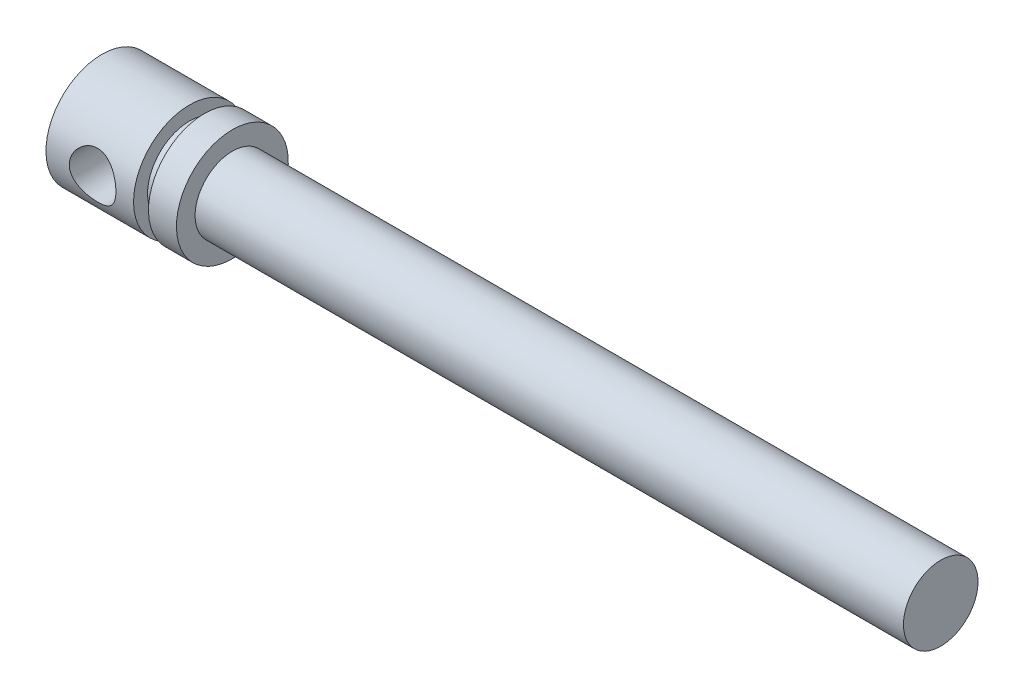
ISO-10303-21;
HEADER;
FILE_DESCRIPTION(('STEP AP214'),'2;1');
FILE_NAME('part.step','',(''),(''),'','','');
FILE_SCHEMA(('AUTOMOTIVE_DESIGN { 1 0 10303 214 1 1 1 1 }'));
ENDSEC;
DATA;
#1=APPLICATION_CONTEXT('core data for automotive mechanical design processes');
#2=APPLICATION_PROTOCOL_DEFINITION('international standard','automotive_design',2000,#1);
#3=PRODUCT_CONTEXT('',#1,'mechanical');
#4=PRODUCT('Part','Part','',(#3));
#5=PRODUCT_RELATED_PRODUCT_CATEGORY('part','',(#4));
#6=PRODUCT_DEFINITION_FORMATION('','',#4);
#7=PRODUCT_DEFINITION_CONTEXT('part definition',#1,'design');
#8=PRODUCT_DEFINITION('design','',#6,#7);
#9=PRODUCT_DEFINITION_SHAPE('','',#8);
#10=(LENGTH_UNIT() NAMED_UNIT(*) SI_UNIT(.MILLI.,.METRE.));
#11=(NAMED_UNIT(*) PLANE_ANGLE_UNIT() SI_UNIT($,.RADIAN.));
#12=(NAMED_UNIT(*) SI_UNIT($,.STERADIAN.) SOLID_ANGLE_UNIT());
#13=UNCERTAINTY_MEASURE_WITH_UNIT(LENGTH_MEASURE(1.E-05),#10,'distance_accuracy_value','');
#14=(GEOMETRIC_REPRESENTATION_CONTEXT(3) GLOBAL_UNCERTAINTY_ASSIGNED_CONTEXT((#13)) GLOBAL_UNIT_ASSIGNED_CONTEXT((#10,
#11,#12)) REPRESENTATION_CONTEXT('',''));
#15=CARTESIAN_POINT('',(0.,0.,0.));
#16=DIRECTION('',(0.,0.,1.));
#17=DIRECTION('',(1.,0.,0.));
#18=AXIS2_PLACEMENT_3D('',#15,#16,#17);
#19=CARTESIAN_POINT('',(0.,0.,0.));
#20=DIRECTION('',(-1.,0.,0.));
#21=DIRECTION('',(0.,-1.,0.));
#22=AXIS2_PLACEMENT_3D('',#19,#20,#21);
#23=PLANE('',#22);
#24=CARTESIAN_POINT('',(0.,0.,0.));
#25=DIRECTION('',(1.,0.,0.));
#26=DIRECTION('',(0.,1.,0.));
#27=AXIS2_PLACEMENT_3D('',#24,#25,#26);
#28=CIRCLE('',#27,6.);
#29=CARTESIAN_POINT('',(0.,6.,0.));
#30=VERTEX_POINT('',#29);
#31=EDGE_CURVE('E51',#30,#30,#28,.T.);
#32=ORIENTED_EDGE('',*,*,#31,.F.);
#33=EDGE_LOOP('',(#32));
#34=FACE_BOUND('',#33,.T.);
#35=ADVANCED_FACE('F40',(#34),#23,.T.);
#36=CARTESIAN_POINT('',(90.,0.,0.));
#37=DIRECTION('',(1.,0.,0.));
#38=DIRECTION('',(0.,1.,0.));
#39=AXIS2_PLACEMENT_3D('',#36,#37,#38);
#40=CYLINDRICAL_SURFACE('',#39,5.99999999999999);
#41=CARTESIAN_POINT('',(7.5,0.,-5.99999999999999));
#42=CARTESIAN_POINT('',(7.4999952878604,-0.133903918163791,-5.99999628290906));
#43=CARTESIAN_POINT('',(7.48917868439947,-0.268039524991424,-5.99546656821163));
#44=CARTESIAN_POINT('',(7.44631926190637,-0.532498019991114,-5.97780115788616));
#45=CARTESIAN_POINT('',(7.41422105321848,-0.66281002980867,-5.9646430059979));
#46=CARTESIAN_POINT('',(7.3301785119407,-0.915376593299225,-5.93112629106011));
#47=CARTESIAN_POINT('',(7.27830140767691,-1.03765681434384,-5.91079213642028));
#48=CARTESIAN_POINT('',(7.15645416697814,-1.27165974779733,-5.86490559253449));
#49=CARTESIAN_POINT('',(7.08648951102523,-1.38338564416287,-5.83935478441346));
#50=CARTESIAN_POINT('',(6.92674208819245,-1.59889674004597,-5.78415660619863));
#51=CARTESIAN_POINT('',(6.83619739674829,-1.70208251703042,-5.75437507703431));
#52=CARTESIAN_POINT('',(6.63947131609954,-1.8923196601971,-5.69465427085227));
#53=CARTESIAN_POINT('',(6.53328174628491,-1.9793625312399,-5.66471491925557));
#54=CARTESIAN_POINT('',(6.30194644898946,-2.13907474876483,-5.60642043928223));
#55=CARTESIAN_POINT('',(6.17612510424857,-2.2108261616941,-5.57821573827598));
#56=CARTESIAN_POINT('',(5.91285348305705,-2.331878813161,-5.52871144633221));
#57=CARTESIAN_POINT('',(5.77540924074289,-2.38119161708799,-5.507408299805));
#58=CARTESIAN_POINT('',(5.49969261673848,-2.45349196589845,-5.47557110795536));
#59=CARTESIAN_POINT('',(5.36177903328898,-2.47763315746001,-5.4645677530895));
#60=CARTESIAN_POINT('',(5.08345341455361,-2.50250419944798,-5.45322652433632));
#61=CARTESIAN_POINT('',(4.94304279992962,-2.5032469611117,-5.45288276849132));
#62=CARTESIAN_POINT('',(4.67519987914757,-2.48216900725155,-5.46250239122984));
#63=CARTESIAN_POINT('',(4.54759780687576,-2.46207362224014,-5.47167765447588));
#64=CARTESIAN_POINT('',(4.29777581799454,-2.40278382032141,-5.49796965547248));
#65=CARTESIAN_POINT('',(4.17555693701519,-2.36358574574513,-5.51508791407033));
#66=CARTESIAN_POINT('',(3.93688459401841,-2.26643917454979,-5.55572369545607));
#67=CARTESIAN_POINT('',(3.82060915817359,-2.20810943078428,-5.57936963898297));
#68=CARTESIAN_POINT('',(3.59904453223936,-2.07462485161169,-5.63036662282145));
#69=CARTESIAN_POINT('',(3.49375969877287,-1.99946338103921,-5.65771912259551));
#70=CARTESIAN_POINT('',(3.28780008253443,-1.82699193108754,-5.71585953755965));
#71=CARTESIAN_POINT('',(3.18826686522916,-1.72834696641502,-5.74674242808946));
#72=CARTESIAN_POINT('',(3.00677299408161,-1.51545918210306,-5.80651346225055));
#73=CARTESIAN_POINT('',(2.92481645661564,-1.40121271889692,-5.83540113754018));
#74=CARTESIAN_POINT('',(2.77912835276747,-1.15689589738674,-5.88876567112945));
#75=CARTESIAN_POINT('',(2.71586110969864,-1.02652116489536,-5.91312533086666));
#76=CARTESIAN_POINT('',(2.61255772079348,-0.755704805053667,-5.95378962829605));
#77=CARTESIAN_POINT('',(2.57250873611237,-0.615268789590071,-5.97009871691599));
#78=CARTESIAN_POINT('',(2.51916801574673,-0.337856226692456,-5.99199282372769));
#79=CARTESIAN_POINT('',(2.5043442851125,-0.201222570557278,-5.99819082094249));
#80=CARTESIAN_POINT('',(2.49730755277181,0.0727093109921778,-6.00112100737489));
#81=CARTESIAN_POINT('',(2.505088059496,0.21000733430527,-5.99785591423877));
#82=CARTESIAN_POINT('',(2.54194216961213,0.474196484682871,-5.98262435313879));
#83=CARTESIAN_POINT('',(2.56993990819439,0.601265933278776,-5.97109774567978));
#84=CARTESIAN_POINT('',(2.64493638908157,0.848765497942179,-5.94097213544828));
#85=CARTESIAN_POINT('',(2.69193753190061,0.969194773036713,-5.92237223919407));
#86=CARTESIAN_POINT('',(2.80514195142423,1.20421799973828,-5.8791654129033));
#87=CARTESIAN_POINT('',(2.87189636629204,1.31851447371068,-5.8543898293856));
#88=CARTESIAN_POINT('',(3.02210675558342,1.53469243246282,-5.80147609158182));
#89=CARTESIAN_POINT('',(3.10556970305865,1.63656870520375,-5.77333653537472));
#90=CARTESIAN_POINT('',(3.29380646654471,1.83266686054867,-5.71424175790866));
#91=CARTESIAN_POINT('',(3.39967700597211,1.92582139596023,-5.68322903182027));
#92=CARTESIAN_POINT('',(3.6260425518712,2.09333969221046,-5.62368673536039));
#93=CARTESIAN_POINT('',(3.74654087034502,2.16769918571027,-5.59515772986986));
#94=CARTESIAN_POINT('',(4.00122835060358,2.2963192041761,-5.54362772487863));
#95=CARTESIAN_POINT('',(4.13558807102375,2.35027836475451,-5.52071125109801));
#96=CARTESIAN_POINT('',(4.41274118762612,2.43434827902353,-5.48416711318334));
#97=CARTESIAN_POINT('',(4.55552752498876,2.46447869724417,-5.47053179113072));
#98=CARTESIAN_POINT('',(4.83363739837805,2.49808160700532,-5.45526329073079));
#99=CARTESIAN_POINT('',(4.96868932451195,2.50342760836084,-5.45278701929113));
#100=CARTESIAN_POINT('',(5.23768572235548,2.49231151038,-5.45787706027258));
#101=CARTESIAN_POINT('',(5.3716303609001,2.47585275892879,-5.46544183100006));
#102=CARTESIAN_POINT('',(5.62818549467776,2.42316809595844,-5.48899102586043));
#103=CARTESIAN_POINT('',(5.75103334597753,2.38789807270203,-5.50456709625452));
#104=CARTESIAN_POINT('',(5.98909604366397,2.29952656276963,-5.54206362465903));
#105=CARTESIAN_POINT('',(6.10430873433601,2.24642006560089,-5.56398586515028));
#106=CARTESIAN_POINT('',(6.33139178814705,2.1202057237392,-5.61333908853253));
#107=CARTESIAN_POINT('',(6.44264464594781,2.04608723750136,-5.64102204404078));
#108=CARTESIAN_POINT('',(6.65172029311513,1.88136812596239,-5.69807379131313));
#109=CARTESIAN_POINT('',(6.74953840503241,1.79076178563715,-5.72744316520043));
#110=CARTESIAN_POINT('',(6.93629730561753,1.58780416898838,-5.78712781593092));
#111=CARTESIAN_POINT('',(7.0240726428278,1.47434977868814,-5.81735619175009));
#112=CARTESIAN_POINT('',(7.17939913004211,1.23319985958043,-5.87320303099821));
#113=CARTESIAN_POINT('',(7.24694106399683,1.1054978774169,-5.89881939160171));
#114=CARTESIAN_POINT('',(7.3584188704516,0.841465213422193,-5.94218308378895));
#115=CARTESIAN_POINT('',(7.40272649429008,0.705312056415867,-5.96005349044658));
#116=CARTESIAN_POINT('',(7.46741568752959,0.426816782070268,-5.98642234975889));
#117=CARTESIAN_POINT('',(7.48787216820581,0.284495506121989,-5.99495014042421));
#118=CARTESIAN_POINT('',(7.49732384178621,0.118052512349437,-5.99888566614291));
#119=CARTESIAN_POINT('',(7.49832660250302,0.0944569348794029,-5.99930292614997));
#120=CARTESIAN_POINT('',(7.49966509825678,0.0472433090693365,-5.99986042138655));
#121=CARTESIAN_POINT('',(7.50000083138364,0.0236252606651506,-6.00000065582279));
#122=CARTESIAN_POINT('',(7.5,0.,-5.99999999999999));
#123=B_SPLINE_CURVE_WITH_KNOTS('',3,(#41,#42,#43,#44,#45,#46,#47,#48,#49,#50,#51,#52,#53,#54,
#55,#56,#57,#58,#59,#60,#61,#62,#63,#64,#65,#66,#67,#68,#69,#70,#71,#72,#73,#74,#75,#76,#77,#78,
#79,#80,#81,#82,#83,#84,#85,#86,#87,#88,#89,#90,#91,#92,#93,#94,#95,#96,#97,#98,#99,#100,#101,
#102,#103,#104,#105,#106,#107,#108,#109,#110,#111,#112,#113,#114,#115,#116,#117,#118,#119,#120,
#121,#122),.UNSPECIFIED.,.T.,.F.,(4,2,2,2,2,2,2,2,2,2,2,2,2,2,2,2,2,2,2,2,2,2,2,2,2,2,2,2,2,2,2,
2,2,2,2,2,2,2,2,2,4),(0.,0.401613837767878,0.804277081257394,1.2055837038126,1.60676887370595,
2.02635872577614,2.44616876262931,2.88663449078251,3.32687293461176,3.74590546275115,
4.16470676498092,4.55140314405113,4.93817359454425,5.33317426117429,5.72833091434413,
6.15688282255793,6.58553498629176,7.02408110121627,7.46238448436594,7.87296886786502,
8.28343534986344,8.67353179471443,9.0636775320357,9.46594270544322,9.86837610938992,
10.2995697605859,10.7308612248068,11.1682957671905,11.6053689414916,12.0087975511929,
12.4121642259507,12.7967529992953,13.1814498990123,13.5892778679488,13.9972474685189,
14.4349307000978,14.8728129885717,15.3034571163877,15.7327450093864,15.8036033125922,
15.8744618187069),.UNSPECIFIED.);
#124=CARTESIAN_POINT('',(7.5,0.,-5.99999999999999));
#125=VERTEX_POINT('',#124);
#126=EDGE_CURVE('E10',#125,#125,#123,.T.);
#127=ORIENTED_EDGE('',*,*,#126,.F.);
#128=EDGE_LOOP('',(#127));
#129=FACE_BOUND('',#128,.T.);
#130=CARTESIAN_POINT('',(7.5,0.,6.));
#131=CARTESIAN_POINT('',(7.4999952878604,0.133903918163793,5.99999628290908));
#132=CARTESIAN_POINT('',(7.48917868439947,0.268039524991427,5.99546656821164));
#133=CARTESIAN_POINT('',(7.44631926190637,0.532498019991115,5.97780115788615));
#134=CARTESIAN_POINT('',(7.41422105321848,0.662810029808672,5.9646430059979));
#135=CARTESIAN_POINT('',(7.3301785119407,0.915376593299227,5.93112629106011));
#136=CARTESIAN_POINT('',(7.27830140767691,1.03765681434384,5.91079213642028));
#137=CARTESIAN_POINT('',(7.15645416697814,1.27165974779733,5.86490559253449));
#138=CARTESIAN_POINT('',(7.08648951102523,1.38338564416287,5.83935478441346));
#139=CARTESIAN_POINT('',(6.92674208819245,1.59889674004597,5.78415660619863));
#140=CARTESIAN_POINT('',(6.83619739674829,1.70208251703042,5.75437507703432));
#141=CARTESIAN_POINT('',(6.63947131609954,1.8923196601971,5.69465427085227));
#142=CARTESIAN_POINT('',(6.53328174628491,1.9793625312399,5.66471491925557));
#143=CARTESIAN_POINT('',(6.30194644898946,2.13907474876483,5.60642043928223));
#144=CARTESIAN_POINT('',(6.17612510424856,2.2108261616941,5.57821573827598));
#145=CARTESIAN_POINT('',(5.91285348305705,2.331878813161,5.52871144633221));
#146=CARTESIAN_POINT('',(5.77540924074289,2.38119161708799,5.507408299805));
#147=CARTESIAN_POINT('',(5.49969261673848,2.45349196589845,5.47557110795536));
#148=CARTESIAN_POINT('',(5.36177903328898,2.47763315746001,5.46456775308951));
#149=CARTESIAN_POINT('',(5.08345341455361,2.50250419944798,5.45322652433632));
#150=CARTESIAN_POINT('',(4.94304279992962,2.5032469611117,5.45288276849132));
#151=CARTESIAN_POINT('',(4.67519987914757,2.48216900725155,5.46250239122984));
#152=CARTESIAN_POINT('',(4.54759780687576,2.46207362224014,5.47167765447588));
#153=CARTESIAN_POINT('',(4.29777581799454,2.40278382032141,5.49796965547248));
#154=CARTESIAN_POINT('',(4.17555693701519,2.36358574574513,5.51508791407033));
#155=CARTESIAN_POINT('',(3.93688459401841,2.26643917454979,5.55572369545607));
#156=CARTESIAN_POINT('',(3.82060915817359,2.20810943078428,5.57936963898297));
#157=CARTESIAN_POINT('',(3.59904453223936,2.07462485161168,5.63036662282145));
#158=CARTESIAN_POINT('',(3.49375969877287,1.99946338103921,5.65771912259551));
#159=CARTESIAN_POINT('',(3.28780008253443,1.82699193108754,5.71585953755965));
#160=CARTESIAN_POINT('',(3.18826686522915,1.72834696641502,5.74674242808946));
#161=CARTESIAN_POINT('',(3.00677299408161,1.51545918210306,5.80651346225055));
#162=CARTESIAN_POINT('',(2.92481645661564,1.40121271889692,5.83540113754018));
#163=CARTESIAN_POINT('',(2.77912835276747,1.15689589738674,5.88876567112945));
#164=CARTESIAN_POINT('',(2.71586110969864,1.02652116489536,5.91312533086666));
#165=CARTESIAN_POINT('',(2.61255772079348,0.755704805053666,5.95378962829606));
#166=CARTESIAN_POINT('',(2.57250873611237,0.61526878959007,5.97009871691599));
#167=CARTESIAN_POINT('',(2.51916801574673,0.337856226692455,5.99199282372769));
#168=CARTESIAN_POINT('',(2.5043442851125,0.201222570557277,5.99819082094249));
#169=CARTESIAN_POINT('',(2.49730755277181,-0.0727093109921785,6.00112100737488));
#170=CARTESIAN_POINT('',(2.505088059496,-0.210007334305271,5.99785591423877));
#171=CARTESIAN_POINT('',(2.54194216961213,-0.474196484682871,5.98262435313879));
#172=CARTESIAN_POINT('',(2.56993990819439,-0.601265933278776,5.97109774567978));
#173=CARTESIAN_POINT('',(2.64493638908157,-0.848765497942179,5.94097213544828));
#174=CARTESIAN_POINT('',(2.69193753190061,-0.969194773036713,5.92237223919407));
#175=CARTESIAN_POINT('',(2.80514195142423,-1.20421799973828,5.8791654129033));
#176=CARTESIAN_POINT('',(2.87189636629204,-1.31851447371069,5.8543898293856));
#177=CARTESIAN_POINT('',(3.02210675558342,-1.53469243246282,5.80147609158181));
#178=CARTESIAN_POINT('',(3.10556970305865,-1.63656870520375,5.77333653537472));
#179=CARTESIAN_POINT('',(3.29380646654471,-1.83266686054867,5.71424175790866));
#180=CARTESIAN_POINT('',(3.39967700597211,-1.92582139596023,5.68322903182027));
#181=CARTESIAN_POINT('',(3.6260425518712,-2.09333969221046,5.62368673536039));
#182=CARTESIAN_POINT('',(3.74654087034502,-2.16769918571027,5.59515772986986));
#183=CARTESIAN_POINT('',(4.00122835060358,-2.2963192041761,5.54362772487863));
#184=CARTESIAN_POINT('',(4.13558807102375,-2.35027836475451,5.52071125109801));
#185=CARTESIAN_POINT('',(4.41274118762612,-2.43434827902353,5.48416711318333));
#186=CARTESIAN_POINT('',(4.55552752498876,-2.46447869724417,5.47053179113072));
#187=CARTESIAN_POINT('',(4.83363739837806,-2.49808160700532,5.45526329073078));
#188=CARTESIAN_POINT('',(4.96868932451195,-2.50342760836084,5.45278701929112));
#189=CARTESIAN_POINT('',(5.23768572235548,-2.49231151038,5.45787706027258));
#190=CARTESIAN_POINT('',(5.3716303609001,-2.47585275892879,5.46544183100006));
#191=CARTESIAN_POINT('',(5.62818549467776,-2.42316809595844,5.48899102586043));
#192=CARTESIAN_POINT('',(5.75103334597753,-2.38789807270203,5.50456709625452));
#193=CARTESIAN_POINT('',(5.98909604366397,-2.29952656276963,5.54206362465903));
#194=CARTESIAN_POINT('',(6.10430873433601,-2.24642006560089,5.56398586515027));
#195=CARTESIAN_POINT('',(6.33139178814705,-2.1202057237392,5.61333908853253));
#196=CARTESIAN_POINT('',(6.44264464594781,-2.04608723750136,5.64102204404078));
#197=CARTESIAN_POINT('',(6.65172029311513,-1.88136812596239,5.69807379131313));
#198=CARTESIAN_POINT('',(6.74953840503241,-1.79076178563715,5.72744316520042));
#199=CARTESIAN_POINT('',(6.93629730561753,-1.58780416898838,5.78712781593091));
#200=CARTESIAN_POINT('',(7.0240726428278,-1.47434977868813,5.81735619175008));
#201=CARTESIAN_POINT('',(7.17939913004211,-1.23319985958043,5.8732030309982));
#202=CARTESIAN_POINT('',(7.24694106399683,-1.1054978774169,5.89881939160171));
#203=CARTESIAN_POINT('',(7.3584188704516,-0.841465213422193,5.94218308378895));
#204=CARTESIAN_POINT('',(7.40272649429008,-0.705312056415867,5.96005349044658));
#205=CARTESIAN_POINT('',(7.46741568752959,-0.426816782070268,5.98642234975889));
#206=CARTESIAN_POINT('',(7.48787216820581,-0.284495506121989,5.99495014042422));
#207=CARTESIAN_POINT('',(7.49732384178621,-0.118052512349436,5.99888566614291));
#208=CARTESIAN_POINT('',(7.49832660250302,-0.0944569348794013,5.99930292614997));
#209=CARTESIAN_POINT('',(7.49966509825678,-0.047243309069334,5.99986042138655));
#210=CARTESIAN_POINT('',(7.50000083138364,-0.0236252606651478,6.00000065582279));
#211=CARTESIAN_POINT('',(7.5,0.,6.));
#212=B_SPLINE_CURVE_WITH_KNOTS('',3,(#130,#131,#132,#133,#134,#135,#136,#137,#138,#139,#140,
#141,#142,#143,#144,#145,#146,#147,#148,#149,#150,#151,#152,#153,#154,#155,#156,#157,#158,#159,
#160,#161,#162,#163,#164,#165,#166,#167,#168,#169,#170,#171,#172,#173,#174,#175,#176,#177,#178,
#179,#180,#181,#182,#183,#184,#185,#186,#187,#188,#189,#190,#191,#192,#193,#194,#195,#196,#197,
#198,#199,#200,#201,#202,#203,#204,#205,#206,#207,#208,#209,#210,#211),.UNSPECIFIED.,.T.,.F.,(4,
2,2,2,2,2,2,2,2,2,2,2,2,2,2,2,2,2,2,2,2,2,2,2,2,2,2,2,2,2,2,2,2,2,2,2,2,2,2,2,4),(0.,
0.401613837767877,0.804277081257393,1.2055837038126,1.60676887370595,2.02635872577614,
2.44616876262931,2.88663449078251,3.32687293461176,3.74590546275115,4.16470676498092,
4.55140314405113,4.93817359454425,5.33317426117429,5.72833091434413,6.15688282255793,
6.58553498629176,7.02408110121626,7.46238448436594,7.87296886786502,8.28343534986344,
8.67353179471443,9.0636775320357,9.46594270544322,9.86837610938992,10.2995697605859,
10.7308612248068,11.1682957671905,11.6053689414916,12.0087975511929,12.4121642259507,
12.7967529992953,13.1814498990123,13.5892778679488,13.9972474685189,14.4349307000978,
14.8728129885716,15.3034571163877,15.7327450093864,15.8036033125922,15.8744618187069),.UNSPECIFIED.);
#213=CARTESIAN_POINT('',(7.5,0.,6.));
#214=VERTEX_POINT('',#213);
#215=EDGE_CURVE('E50',#214,#214,#212,.T.);
#216=ORIENTED_EDGE('',*,*,#215,.F.);
#217=EDGE_LOOP('',(#216));
#218=FACE_BOUND('',#217,.T.);
#219=ORIENTED_EDGE('',*,*,#31,.T.);
#220=EDGE_LOOP('',(#219));
#221=FACE_BOUND('',#220,.T.);
#222=CARTESIAN_POINT('',(9.39999999999999,0.,0.));
#223=DIRECTION('',(1.,0.,0.));
#224=DIRECTION('',(0.,1.,0.));
#225=AXIS2_PLACEMENT_3D('',#222,#223,#224);
#226=CIRCLE('',#225,5.99999999999998);
#227=CARTESIAN_POINT('',(9.39999999999999,5.99999999999999,0.));
#228=VERTEX_POINT('',#227);
#229=EDGE_CURVE('E54',#228,#228,#226,.T.);
#230=ORIENTED_EDGE('',*,*,#229,.F.);
#231=EDGE_LOOP('',(#230));
#232=FACE_BOUND('',#231,.T.);
#233=ADVANCED_FACE('F63',(#129,#218,#221,#232),#40,.T.);
#234=CARTESIAN_POINT('',(9.4,5.99999999999999,0.));
#235=DIRECTION('',(1.,0.,0.));
#236=DIRECTION('',(0.,1.,0.));
#237=AXIS2_PLACEMENT_3D('',#234,#235,#236);
#238=PLANE('',#237);
#239=ORIENTED_EDGE('',*,*,#229,.T.);
#240=EDGE_LOOP('',(#239));
#241=FACE_BOUND('',#240,.T.);
#242=CARTESIAN_POINT('',(9.39999999999999,0.,0.));
#243=DIRECTION('',(1.,0.,0.));
#244=DIRECTION('',(0.,1.,0.));
#245=AXIS2_PLACEMENT_3D('',#242,#243,#244);
#246=CIRCLE('',#245,4.49999999999999);
#247=CARTESIAN_POINT('',(9.39999999999999,4.49999999999999,0.));
#248=VERTEX_POINT('',#247);
#249=EDGE_CURVE('E108',#248,#248,#246,.T.);
#250=ORIENTED_EDGE('',*,*,#249,.F.);
#251=EDGE_LOOP('',(#250));
#252=FACE_BOUND('',#251,.T.);
#253=ADVANCED_FACE('F93',(#241,#252),#238,.T.);
#254=CARTESIAN_POINT('',(90.,0.,0.));
#255=DIRECTION('',(1.,0.,0.));
#256=DIRECTION('',(0.,1.,0.));
#257=AXIS2_PLACEMENT_3D('',#254,#255,#256);
#258=CYLINDRICAL_SURFACE('',#257,4.49999999999998);
#259=ORIENTED_EDGE('',*,*,#249,.T.);
#260=EDGE_LOOP('',(#259));
#261=FACE_BOUND('',#260,.T.);
#262=CARTESIAN_POINT('',(11.,0.,0.));
#263=DIRECTION('',(1.,0.,0.));
#264=DIRECTION('',(0.,1.,0.));
#265=AXIS2_PLACEMENT_3D('',#262,#263,#264);
#266=CIRCLE('',#265,4.49999999999998);
#267=CARTESIAN_POINT('',(11.,4.49999999999999,0.));
#268=VERTEX_POINT('',#267);
#269=EDGE_CURVE('E112',#268,#268,#266,.T.);
#270=ORIENTED_EDGE('',*,*,#269,.F.);
#271=EDGE_LOOP('',(#270));
#272=FACE_BOUND('',#271,.T.);
#273=ADVANCED_FACE('F86',(#261,#272),#258,.T.);
#274=CARTESIAN_POINT('',(11.,4.49999999999999,0.));
#275=DIRECTION('',(-1.,0.,0.));
#276=DIRECTION('',(0.,-1.,0.));
#277=AXIS2_PLACEMENT_3D('',#274,#275,#276);
#278=PLANE('',#277);
#279=ORIENTED_EDGE('',*,*,#269,.T.);
#280=EDGE_LOOP('',(#279));
#281=FACE_BOUND('',#280,.T.);
#282=CARTESIAN_POINT('',(11.,0.,0.));
#283=DIRECTION('',(1.,0.,0.));
#284=DIRECTION('',(0.,1.,0.));
#285=AXIS2_PLACEMENT_3D('',#282,#283,#284);
#286=CIRCLE('',#285,5.99999999999998);
#287=CARTESIAN_POINT('',(11.,5.99999999999999,0.));
#288=VERTEX_POINT('',#287);
#289=EDGE_CURVE('E118',#288,#288,#286,.T.);
#290=ORIENTED_EDGE('',*,*,#289,.F.);
#291=EDGE_LOOP('',(#290));
#292=FACE_BOUND('',#291,.T.);
#293=ADVANCED_FACE('F83',(#281,#292),#278,.T.);
#294=CARTESIAN_POINT('',(90.,0.,0.));
#295=DIRECTION('',(1.,0.,0.));
#296=DIRECTION('',(0.,1.,0.));
#297=AXIS2_PLACEMENT_3D('',#294,#295,#296);
#298=CYLINDRICAL_SURFACE('',#297,5.99999999999998);
#299=ORIENTED_EDGE('',*,*,#289,.T.);
#300=EDGE_LOOP('',(#299));
#301=FACE_BOUND('',#300,.T.);
#302=CARTESIAN_POINT('',(14.,0.,0.));
#303=DIRECTION('',(1.,0.,0.));
#304=DIRECTION('',(0.,1.,0.));
#305=AXIS2_PLACEMENT_3D('',#302,#303,#304);
#306=CIRCLE('',#305,5.99999999999998);
#307=CARTESIAN_POINT('',(14.,5.99999999999999,0.));
#308=VERTEX_POINT('',#307);
#309=EDGE_CURVE('E120',#308,#308,#306,.T.);
#310=ORIENTED_EDGE('',*,*,#309,.F.);
#311=EDGE_LOOP('',(#310));
#312=FACE_BOUND('',#311,.T.);
#313=ADVANCED_FACE('F76',(#301,#312),#298,.T.);
#314=CARTESIAN_POINT('',(14.,5.99999999999999,0.));
#315=DIRECTION('',(1.,0.,0.));
#316=DIRECTION('',(0.,1.,0.));
#317=AXIS2_PLACEMENT_3D('',#314,#315,#316);
#318=PLANE('',#317);
#319=ORIENTED_EDGE('',*,*,#309,.T.);
#320=EDGE_LOOP('',(#319));
#321=FACE_BOUND('',#320,.T.);
#322=CARTESIAN_POINT('',(14.,0.,0.));
#323=DIRECTION('',(1.,0.,0.));
#324=DIRECTION('',(0.,1.,0.));
#325=AXIS2_PLACEMENT_3D('',#322,#323,#324);
#326=CIRCLE('',#325,3.99999999999998);
#327=CARTESIAN_POINT('',(14.,3.99999999999999,0.));
#328=VERTEX_POINT('',#327);
#329=EDGE_CURVE('E125',#328,#328,#326,.T.);
#330=ORIENTED_EDGE('',*,*,#329,.F.);
#331=EDGE_LOOP('',(#330));
#332=FACE_BOUND('',#331,.T.);
#333=ADVANCED_FACE('F78',(#321,#332),#318,.T.);
#334=CARTESIAN_POINT('',(90.,0.,0.));
#335=DIRECTION('',(1.,0.,0.));
#336=DIRECTION('',(0.,1.,0.));
#337=AXIS2_PLACEMENT_3D('',#334,#335,#336);
#338=CYLINDRICAL_SURFACE('',#337,3.99999999999997);
#339=ORIENTED_EDGE('',*,*,#329,.T.);
#340=EDGE_LOOP('',(#339));
#341=FACE_BOUND('',#340,.T.);
#342=CARTESIAN_POINT('',(90.,0.,0.));
#343=DIRECTION('',(1.,0.,0.));
#344=DIRECTION('',(0.,1.,0.));
#345=AXIS2_PLACEMENT_3D('',#342,#343,#344);
#346=CIRCLE('',#345,3.99999999999996);
#347=CARTESIAN_POINT('',(90.,4.,0.));
#348=VERTEX_POINT('',#347);
#349=EDGE_CURVE('E124',#348,#348,#346,.T.);
#350=ORIENTED_EDGE('',*,*,#349,.F.);
#351=EDGE_LOOP('',(#350));
#352=FACE_BOUND('',#351,.T.);
#353=ADVANCED_FACE('F75',(#341,#352),#338,.T.);
#354=CARTESIAN_POINT('',(90.,4.,0.));
#355=DIRECTION('',(1.,0.,0.));
#356=DIRECTION('',(0.,1.,0.));
#357=AXIS2_PLACEMENT_3D('',#354,#355,#356);
#358=PLANE('',#357);
#359=ORIENTED_EDGE('',*,*,#349,.T.);
#360=EDGE_LOOP('',(#359));
#361=FACE_BOUND('',#360,.T.);
#362=ADVANCED_FACE('F67',(#361),#358,.T.);
#363=CARTESIAN_POINT('',(5.,0.,-6.));
#364=DIRECTION('',(0.,0.,1.));
#365=DIRECTION('',(1.,0.,0.));
#366=AXIS2_PLACEMENT_3D('',#363,#364,#365);
#367=CYLINDRICAL_SURFACE('',#366,2.5);
#368=ORIENTED_EDGE('',*,*,#126,.T.);
#369=EDGE_LOOP('',(#368));
#370=FACE_BOUND('',#369,.T.);
#371=ORIENTED_EDGE('',*,*,#215,.T.);
#372=EDGE_LOOP('',(#371));
#373=FACE_BOUND('',#372,.T.);
#374=ADVANCED_FACE('F65',(#370,#373),#367,.F.);
#375=CLOSED_SHELL('',(#35,#233,#253,#273,#293,#313,#333,#353,#362,#374));
#376=MANIFOLD_SOLID_BREP('B2',#375);
#377=ADVANCED_BREP_SHAPE_REPRESENTATION('',(#18,#376),#14);
#378=SHAPE_DEFINITION_REPRESENTATION(#9,#377);
ENDSEC;
END-ISO-10303-21;
